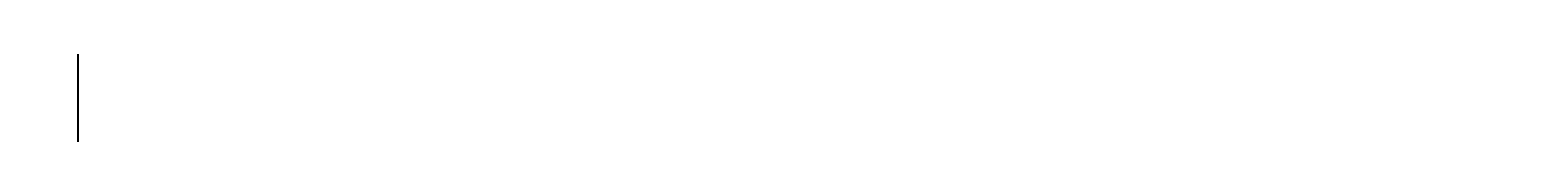
# Model space of a CAD drawing. Units: inches. Extents: x 35362 to 73946, y 43607 to 67532.
# Tile 99 of 134: x 50119 to 50761, y 49269 to 49298. Entities that reach past the tile are written whole.
import ezdxf

# ---------------------------------------------------------------- set-up
doc = ezdxf.new("R2010")
doc.units = ezdxf.units.IN
doc.header["$MEASUREMENT"] = 0
doc.layers.add('A-ANNO-DIMS', color=2, linetype='Continuous', lineweight=18)
doc.styles.get("Standard").update_dxf_attribs({"font": 'arial.ttf'})
doc.dimstyles.get("Standard").update_dxf_attribs({"dimtxt": 0.18, "dimasz": 0.18, "dimexe": 0.18, "dimexo": 0.0625, "dimgap": 0.09, "dimtad": 0, "dimtih": 1, "dimtoh": 1, "dimdec": 4, "dimzin": 0, "dimdsep": 46, "dimtxsty": 'Standard', "dimcen": 0.09, "dimadec": 0, "dimazin": 0, "dimtfac": 1, "dimtdec": 4, "dimtofl": 0, "dimtmove": 0, "dimatfit": 3, "dimfxl": 1, "dimtolj": 1, "dimtzin": 0, "dimarcsym": 0})

# ---------------------------------------------------------------- blocks, each defined once
blk = doc.blocks.new('*D11')
at = {"layer": 'A-ANNO-DIMS', "color": 0, "lineweight": -2, "transparency": 16777216}
for p, q in [((47978.66, 56028.77), (47978.66, 43606.68)), ((53109.76, 56028.77), (53109.76, 43606.68)), ((47978.84, 43606.86), (50543.87, 43606.86)), ((53109.58, 43606.86), (50544.55, 43606.86))]:
    blk.add_line(p, q, dxfattribs=at)
at = {"layer": 'A-ANNO-DIMS', "color": 0, "transparency": 16777216}
for points in [[(47978.84, 43606.89), (47978.84, 43606.83), (47978.66, 43606.86)], [(53109.58, 43606.89), (53109.58, 43606.83), (53109.76, 43606.86)]]:
    blk.add_solid(points, dxfattribs=at)
at = {"layer": 'Defpoints', "color": 0, "transparency": 16777216}
for p in [(47978.66, 56028.84), (53109.76, 56028.84), (53109.76, 43606.86)]:
    blk.add_point(p, dxfattribs=at)
at = {"layer": 'A-ANNO-DIMS', "color": 0, "transparency": 16777216, "insert": (50544.21, 43606.86), "char_height": 0.18, "attachment_point": 5}
blk.add_mtext('\\A1;5131', dxfattribs=at)
blk = doc.blocks.new('*D13')
at = {"layer": 'A-ANNO-DIMS', "color": 0, "lineweight": -2, "transparency": 16777216}
for p, q in [((48373.49, 51694.02), (48373.49, 43606.68)), ((51029.04, 51694.02), (51029.04, 43606.68)), ((48373.67, 43606.86), (49700.8, 43606.86)), ((51028.86, 43606.86), (49701.73, 43606.86))]:
    blk.add_line(p, q, dxfattribs=at)
at = {"layer": 'A-ANNO-DIMS', "color": 0, "transparency": 16777216}
for points in [[(48373.67, 43606.89), (48373.67, 43606.83), (48373.49, 43606.86)], [(51028.86, 43606.89), (51028.86, 43606.83), (51029.04, 43606.86)]]:
    blk.add_solid(points, dxfattribs=at)
at = {"layer": 'Defpoints', "color": 0, "transparency": 16777216}
for p in [(48373.49, 51694.09), (51029.04, 51694.09), (51029.04, 43606.86)]:
    blk.add_point(p, dxfattribs=at)
at = {"layer": 'A-ANNO-DIMS', "color": 0, "transparency": 16777216, "insert": (49701.27, 43606.86), "char_height": 0.18, "attachment_point": 5}
blk.add_mtext('\\A1;2655.6', dxfattribs=at)
blk = doc.blocks.new('*D17')
at = {"layer": 'A-ANNO-DIMS', "color": 0, "lineweight": -2, "transparency": 16777216}
for p, q in [((49923.31, 61293.22), (49923.31, 43606.68)), ((51913.93, 61293.22), (51913.93, 43606.68)), ((49923.49, 43606.86), (50918.16, 43606.86)), ((51913.75, 43606.86), (50919.07, 43606.86))]:
    blk.add_line(p, q, dxfattribs=at)
at = {"layer": 'A-ANNO-DIMS', "color": 0, "transparency": 16777216}
for points in [[(49923.49, 43606.89), (49923.49, 43606.83), (49923.31, 43606.86)], [(51913.75, 43606.89), (51913.75, 43606.83), (51913.93, 43606.86)]]:
    blk.add_solid(points, dxfattribs=at)
at = {"layer": 'Defpoints', "color": 0, "transparency": 16777216}
for p in [(49923.31, 61293.29), (51913.93, 61293.29), (51913.93, 43606.86)]:
    blk.add_point(p, dxfattribs=at)
at = {"layer": 'A-ANNO-DIMS', "color": 0, "transparency": 16777216, "insert": (50918.62, 43606.86), "char_height": 0.18, "attachment_point": 5}
blk.add_mtext('\\A1;1990.6', dxfattribs=at)
blk = doc.blocks.new('*D67')
at = {"layer": 'A-ANNO-DIMS', "color": 0, "lineweight": -2, "transparency": 16777216}
for p, q in [((56873.54, 53351.53), (35361.77, 53351.53)), ((35361.95, 53351.35), (35361.95, 49400.89)), ((35361.95, 45450.07), (35361.95, 49400.53)), ((53793.58, 45449.89), (35361.77, 45449.89))]:
    blk.add_line(p, q, dxfattribs=at)
at = {"layer": 'A-ANNO-DIMS', "color": 0, "transparency": 16777216}
for points in [[(35361.92, 53351.35), (35361.98, 53351.35), (35361.95, 53351.53)], [(35361.92, 45450.07), (35361.98, 45450.07), (35361.95, 45449.89)]]:
    blk.add_solid(points, dxfattribs=at)
at = {"layer": 'Defpoints', "color": 0, "transparency": 16777216}
for p in [(35361.95, 53351.53), (56873.6, 53351.53), (53793.64, 45449.89)]:
    blk.add_point(p, dxfattribs=at)
at = {"layer": 'A-ANNO-DIMS', "color": 0, "transparency": 16777216, "insert": (35361.95, 49400.71), "char_height": 0.18, "attachment_point": 5}
blk.add_mtext('\\A1;7901.6', dxfattribs=at)
blk = doc.blocks.new('*D86')
at = {"layer": 'A-ANNO-DIMS', "color": 0, "lineweight": -2, "transparency": 16777216}
for p, q in [((51285.53, 49320.08), (35361.77, 49320.08)), ((35361.95, 49319.9), (35361.95, 49120.26)), ((35361.95, 48920.26), (35361.95, 49119.9)), ((51285.53, 48920.08), (35361.77, 48920.08))]:
    blk.add_line(p, q, dxfattribs=at)
at = {"layer": 'A-ANNO-DIMS', "color": 0, "transparency": 16777216}
for points in [[(35361.92, 49319.9), (35361.98, 49319.9), (35361.95, 49320.08)], [(35361.92, 48920.26), (35361.98, 48920.26), (35361.95, 48920.08)]]:
    blk.add_solid(points, dxfattribs=at)
at = {"layer": 'Defpoints', "color": 0, "transparency": 16777216}
for p in [(35361.95, 49320.08), (51285.59, 49320.08), (51285.59, 48920.08)]:
    blk.add_point(p, dxfattribs=at)
at = {"layer": 'A-ANNO-DIMS', "color": 0, "transparency": 16777216, "insert": (35361.95, 49120.08), "char_height": 0.18, "attachment_point": 5}
blk.add_mtext('\\A1;400.0', dxfattribs=at)
blk = doc.blocks.new('*D107')
at = {"layer": 'A-ANNO-DIMS', "color": 0, "lineweight": -2, "transparency": 16777216}
for p, q in [((50139.56, 59850.01), (50139.56, 43606.68)), ((51320.81, 59850.01), (51320.81, 43606.68)), ((50139.74, 43606.86), (50729.73, 43606.86)), ((51320.63, 43606.86), (50730.64, 43606.86))]:
    blk.add_line(p, q, dxfattribs=at)
at = {"layer": 'A-ANNO-DIMS', "color": 0, "transparency": 16777216}
for points in [[(50139.74, 43606.89), (50139.74, 43606.83), (50139.56, 43606.86)], [(51320.63, 43606.89), (51320.63, 43606.83), (51320.81, 43606.86)]]:
    blk.add_solid(points, dxfattribs=at)
at = {"layer": 'Defpoints', "color": 0, "transparency": 16777216}
for p in [(50139.56, 59850.08), (51320.81, 59850.08), (51320.81, 43606.86)]:
    blk.add_point(p, dxfattribs=at)
at = {"layer": 'A-ANNO-DIMS', "color": 0, "transparency": 16777216, "insert": (50730.19, 43606.86), "char_height": 0.18, "attachment_point": 5}
blk.add_mtext('\\A1;1181.3', dxfattribs=at)

msp = doc.modelspace()

# ---------------------------------------------------------------- dimensions: what is measured, and where the dimension line sits
at = {"layer": 'A-ANNO-DIMS'}
for base, p1, p2, override, picture, middle in [((51913.931, 43606.859), (49923.307, 61293.286), (51913.931, 61293.286), {"dimdec": 1, "dimlfac": 1, "dimrnd": 0, "dimzin": 0, "dimdsep": 46, "dimlunit": 2}, '*D17', (50918.619, 43606.859)), ((51320.8133, 43606.859), (50139.5627, 59850.0769), (51320.8133, 59850.0769), {"dimdec": 1, "dimlfac": 1, "dimrnd": 0, "dimzin": 0, "dimdsep": 46, "dimlunit": 2}, '*D107', (50730.188, 43606.859)), ((53109.76, 43606.859), (47978.665, 56028.836), (53109.76, 56028.836), {"dimdec": 0, "dimlfac": 1, "dimrnd": 0, "dimzin": 0, "dimdsep": 46, "dimlunit": 2}, '*D11', (50544.212, 43606.859)), ((51029.043, 43606.859), (48373.492, 51694.087), (51029.043, 51694.087), {"dimdec": 1, "dimlfac": 1, "dimrnd": 0, "dimzin": 0, "dimdsep": 46, "dimlunit": 2}, '*D13', (49701.267, 43606.859))]:
    dim = msp.add_linear_dim(base=base, p1=p1, p2=p2, dimstyle='Standard', override=override, dxfattribs=at)
    dim.commit()
    dim.dimension.update_dxf_attribs({"geometry": picture, "text_midpoint": middle})
for base, p1, p2, picture, middle in [((35361.949, 53351.529), (53793.638, 45449.894), (56873.602, 53351.529), '*D67', (35361.949, 49400.712)), ((35361.949, 49320.079), (51285.595, 48920.079), (51285.595, 49320.079), '*D86', (35361.949, 49120.079))]:
    dim = msp.add_linear_dim(base=base, p1=p1, p2=p2, angle=90, dimstyle='Standard', override={"dimdec": 1, "dimlfac": 1, "dimrnd": 0, "dimzin": 0, "dimdsep": 46, "dimlunit": 2}, dxfattribs=at)
    dim.commit()
    dim.dimension.update_dxf_attribs({"geometry": picture, "text_midpoint": middle})

doc.saveas('drawing.dxf')
